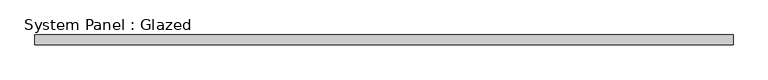
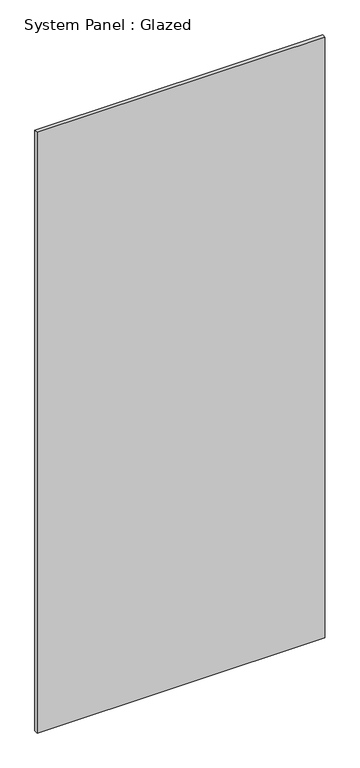
"""IFC4 building model written with IfcOpenShell, lengths in millimetres: plate geometry, System Panel : Glazed."""

from ifc_helpers import new_model, si_unit, origin, origin_with_axes, place, context, project, spatial, polyline, outline, extrude, source, transform, mapped, element, save


def system_panel_glazed_e61de5c1(model_context):
    return source(origin(), model_context, "Body", "SweptSolid", [
        extrude(outline(polyline([(906.2244869, 24.5), (-906.2244869, 24.5), (-906.2244869, 49.5), (906.2244869, 49.5), (906.2244869, 24.5)])), origin_with_axes(), (0.0, 0.0, 1.0), 4000.0),
    ])


if __name__ == "__main__":
    model = new_model("IFC4")
    model_context = context("Model", 3, world=origin())
    ifc_project = project(units=[si_unit("LENGTHUNIT", "METRE", prefix="MILLI")], contexts=[model_context])
    site = spatial("IfcSite", under=ifc_project)
    building = spatial("IfcBuilding", under=site)
    placement = place(None, origin())
    system_panel_glazed_shape = system_panel_glazed_e61de5c1(model_context)
    element("IfcPlate", 1, ObjectType="System Panel : Glazed", at=placement, inside=building, context=model_context, shape_type="MappedRepresentation", body=[
        mapped(system_panel_glazed_shape, transform((0.0, 0.0, 0.0), x_axis=(1.0, 0.0, 0.0), y_axis=(0.0, 1.0, 0.0), z_axis=(0.0, 0.0, 1.0))),
    ])
    save(model, "model.ifc")

# Revit data of these elements
# Type "System Panel : Glazed"
#   Keynote = "H11"
#   Construction Type Id = "GSP4R"
#   Analytic Construction = "1/8 in Pilkington single glazing"
#   Visual Light Transmittance = 0.9
#   Solar Heat Gain Coefficient = 0.86
#   Heat Transfer Coefficient (U) = 6.7069 W/(m²·K)
#   Define Thermal Properties by = 1
# Element 1 (IfcPlate, "System Panel : Glazed")
#   Materials on its faces: "Glass"
# Materials
#   "Glass": class "Glass", colour RGB 0 128 192, transparency 0.9, Description = "Soda Lime Glass", Cost = 0
